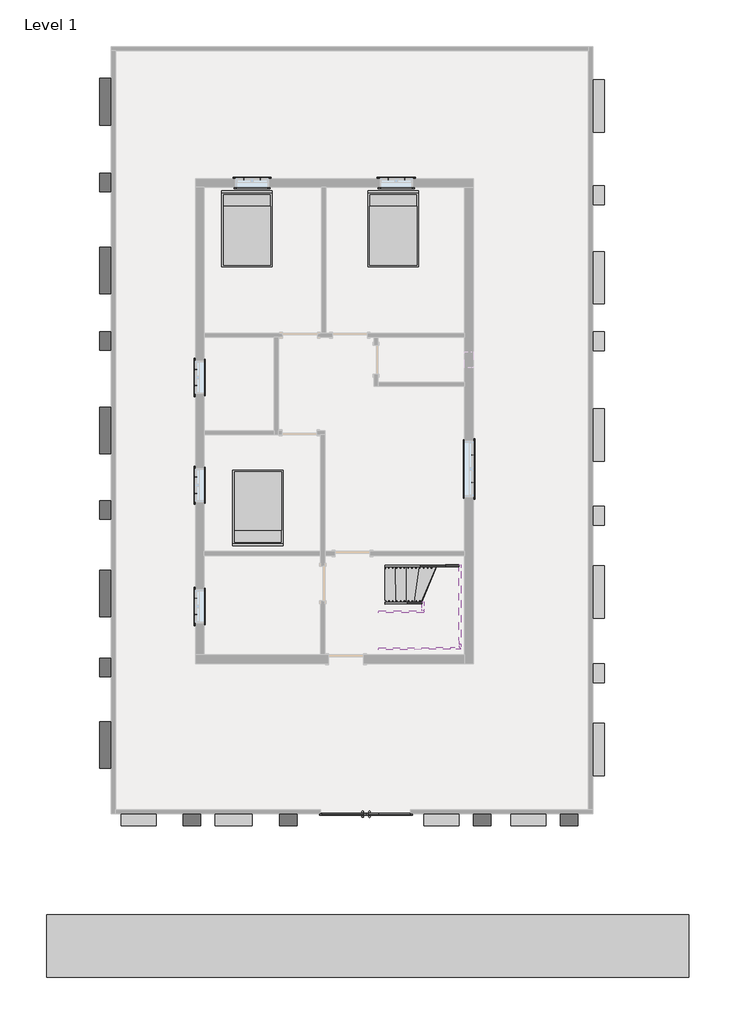
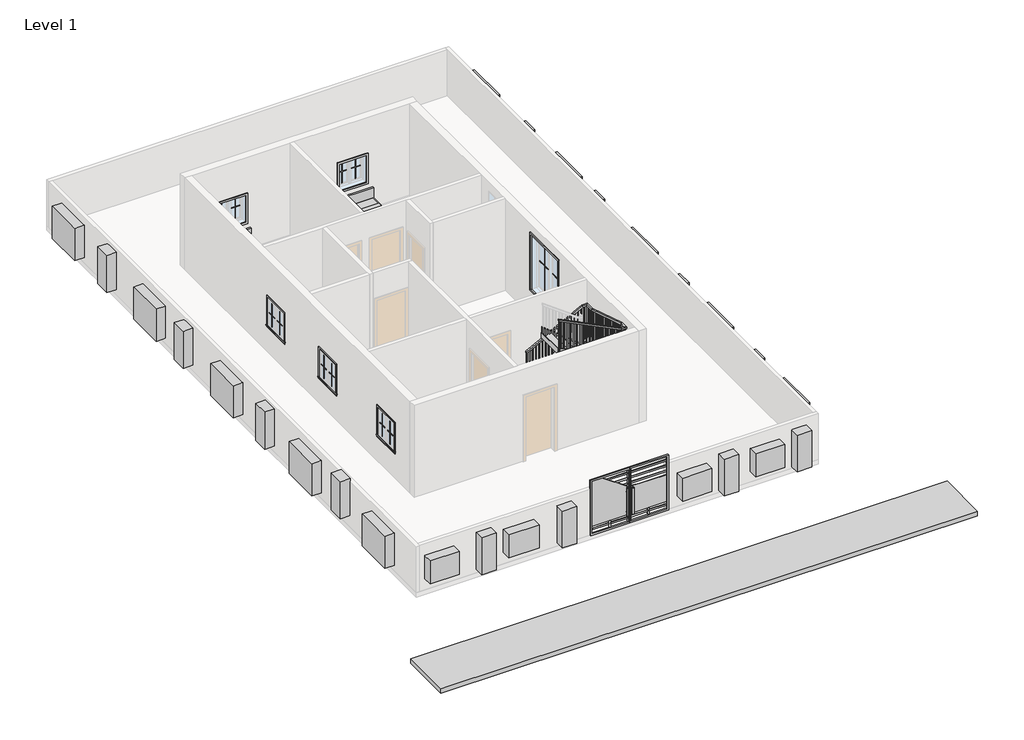
# One storey, part 2 of 2: 30 proxies, 9 members, 3 furniture elements, 1 railing, 1 stair flight.
"""IFC4 building model written with IfcOpenShell, lengths in millimetres."""

from ifc_helpers import new_model, si_unit, frame, origin, place, context, project, spatial, polyline, outline, extrude, faceted_brep, transform, mapped, element, save
from components import generic_models_113f6068, generic_models_1_generic_models_1_f3bdfb45, generic_models_2_generic_models_2_eb82d3b8, generic_models_3_generic_models_3_98a77e8e, generic_models_4_generic_models_4_94af110e, generic_models_6_generic_models_6_790b48f3, muntin_pattern_2x2_muntin_pattern_2x2_b3fe6957, muntin_pattern_2x2_muntin_pattern_2x2_3e0ecaf2, muntin_pattern_2x2_muntin_pattern_2x2_bff912c5, muntin_pattern_2x2_muntin_pattern_2x2_c2194282, trim_window_exterior_flat_with_sill_41619996, trim_window_exterior_flat_with_sill_e04b3088, trim_window_interior_flat_picture_frame_51c85655, trim_window_interior_flat_picture_frame_2a7685fe, bed_17739_bed_17739_15c61121, stair_flight_2f6b2362

model = new_model("IFC4")

# Units and contexts
model_context = context("Model", 3, world=origin())
ifc_project = project(units=[si_unit("LENGTHUNIT", "METRE", prefix="MILLI")], contexts=[model_context])

# Site, building, storey
site = spatial("IfcSite", under=ifc_project)
building = spatial("IfcBuilding", under=site)
storey = spatial("IfcBuildingStorey", under=building, Name="Level 1", Elevation=0.0)

# Proxies
placement = place(None, origin())
generic_models_shape = generic_models_113f6068(model_context)
element("IfcBuildingElementProxy", 1, Name="Generic Models", at=placement, inside=storey, context=model_context, shape_type="MappedRepresentation", body=[
    mapped(generic_models_shape, transform((-423.3915084, -9726.243996, 0.0), x_axis=(1.0, 0.0, 0.0), y_axis=(0.0, 1.0, 0.0), z_axis=(0.0, 0.0, 1.0))),
])
generic_models_1_generic_models_1_shape = generic_models_1_generic_models_1_f3bdfb45(model_context)
element("IfcBuildingElementProxy", 2, Name="Generic Models 1 : Generic Models 1", ObjectType="Generic Models 1 : Generic Models 1", at=placement, inside=storey, context=model_context, shape_type="MappedRepresentation", body=[
    mapped(generic_models_1_generic_models_1_shape, transform((0.0, 0.0, 0.0), x_axis=(1.0, 0.0, 0.0), y_axis=(0.0, 1.0, 0.0), z_axis=(0.0, 0.0, 1.0))),
])
generic_models_2_generic_models_2_shape = generic_models_2_generic_models_2_eb82d3b8(model_context)
element("IfcBuildingElementProxy", 3, Name="Generic Models 2 : Generic Models 2", ObjectType="Generic Models 2 : Generic Models 2", at=placement, inside=storey, context=model_context, shape_type="MappedRepresentation", body=[
    mapped(generic_models_2_generic_models_2_shape, transform((0.0, 0.0, 0.0), x_axis=(1.0, 0.0, 0.0), y_axis=(0.0, 1.0, 0.0), z_axis=(0.0, 0.0, 1.0))),
])
generic_models_3_generic_models_3_shape = generic_models_3_generic_models_3_98a77e8e(model_context)
element("IfcBuildingElementProxy", 4, Name="Generic Models 3 : Generic Models 3", ObjectType="Generic Models 3 : Generic Models 3", at=placement, inside=storey, context=model_context, shape_type="MappedRepresentation", body=[
    mapped(generic_models_3_generic_models_3_shape, transform((0.0, 0.0, 0.0), x_axis=(1.0, 0.0, 0.0), y_axis=(0.0, 1.0, 0.0), z_axis=(0.0, 0.0, 1.0))),
])
generic_models_4_generic_models_4_shape = generic_models_4_generic_models_4_94af110e(model_context)
element("IfcBuildingElementProxy", 5, Name="Generic Models 4 : Generic Models 4", ObjectType="Generic Models 4 : Generic Models 4", at=placement, inside=storey, context=model_context, shape_type="MappedRepresentation", body=[
    mapped(generic_models_4_generic_models_4_shape, transform((0.0, 0.0, 0.0), x_axis=(1.0, 0.0, 0.0), y_axis=(0.0, 1.0, 0.0), z_axis=(0.0, 0.0, 1.0))),
])
generic_models_6_generic_models_6_shape = generic_models_6_generic_models_6_790b48f3(model_context)
element("IfcBuildingElementProxy", 6, Name="Generic Models 6 : Generic Models 6", ObjectType="Generic Models 6 : Generic Models 6", at=placement, inside=storey, context=model_context, shape_type="MappedRepresentation", body=[
    mapped(generic_models_6_generic_models_6_shape, transform((0.0, 0.0, 0.0), x_axis=(1.0, 0.0, 0.0), y_axis=(0.0, 1.0, 0.0), z_axis=(0.0, 0.0, 1.0))),
])
muntin_pattern_2x2_muntin_pattern_2x2_shape = muntin_pattern_2x2_muntin_pattern_2x2_b3fe6957(model_context)
element("IfcBuildingElementProxy", 7, Name="Muntin Pattern_2x2 : Muntin Pattern_2x2", ObjectType="Muntin Pattern_2x2 : Muntin Pattern_2x2", at=placement, inside=storey, context=model_context, shape_type="MappedRepresentation", body=[
    mapped(muntin_pattern_2x2_muntin_pattern_2x2_shape, transform((-3622.2040084, 6872.3185985, 984.25), x_axis=(1.0, 0.0, 0.0), y_axis=(0.0, 1.0, 0.0), z_axis=(0.0, 0.0, 1.0))),
])
element("IfcBuildingElementProxy", 8, Name="Muntin Pattern_2x2 : Muntin Pattern_2x2", ObjectType="Muntin Pattern_2x2 : Muntin Pattern_2x2", at=placement, inside=storey, context=model_context, shape_type="MappedRepresentation", body=[
    mapped(muntin_pattern_2x2_muntin_pattern_2x2_shape, transform((152.8709916, 6872.3185985, 984.25), x_axis=(1.0, 0.0, 0.0), y_axis=(0.0, 1.0, 0.0), z_axis=(0.0, 0.0, 1.0))),
])
element("IfcBuildingElementProxy", 9, Name="Muntin Pattern_2x2 : Muntin Pattern_2x2", ObjectType="Muntin Pattern_2x2 : Muntin Pattern_2x2", at=placement, inside=storey, context=model_context, shape_type="MappedRepresentation", body=[
    mapped(muntin_pattern_2x2_muntin_pattern_2x2_shape, transform((-4884.2665084, 1466.8810985, 984.25), x_axis=(0.0, 1.0, 0.0), y_axis=(-1.0, 0.0, 0.0), z_axis=(0.0, 0.0, 1.0))),
])
element("IfcBuildingElementProxy", 10, Name="Muntin Pattern_2x2 : Muntin Pattern_2x2", ObjectType="Muntin Pattern_2x2 : Muntin Pattern_2x2", at=placement, inside=storey, context=model_context, shape_type="MappedRepresentation", body=[
    mapped(muntin_pattern_2x2_muntin_pattern_2x2_shape, transform((-4884.2665084, -1352.5189015, 984.25), x_axis=(0.0, 1.0, 0.0), y_axis=(-1.0, 0.0, 0.0), z_axis=(0.0, 0.0, 1.0))),
])
element("IfcBuildingElementProxy", 11, Name="Muntin Pattern_2x2 : Muntin Pattern_2x2", ObjectType="Muntin Pattern_2x2 : Muntin Pattern_2x2", at=placement, inside=storey, context=model_context, shape_type="MappedRepresentation", body=[
    mapped(muntin_pattern_2x2_muntin_pattern_2x2_shape, transform((-4884.2665084, -4524.3439015, 984.25), x_axis=(0.0, 1.0, 0.0), y_axis=(-1.0, 0.0, 0.0), z_axis=(0.0, 0.0, 1.0))),
])
muntin_pattern_2x2_muntin_pattern_2x2_2_shape = muntin_pattern_2x2_muntin_pattern_2x2_3e0ecaf2(model_context)
element("IfcBuildingElementProxy", 12, Name="Muntin Pattern_2x2 : Muntin Pattern_2x2", ObjectType="Muntin Pattern_2x2 : Muntin Pattern_2x2", at=placement, inside=storey, context=model_context, shape_type="MappedRepresentation", body=[
    mapped(muntin_pattern_2x2_muntin_pattern_2x2_2_shape, transform((-3193.5790084, 6872.3185985, 984.25), x_axis=(-1.0, 0.0, 0.0), y_axis=(0.0, -1.0, 0.0), z_axis=(0.0, 0.0, 1.0))),
])
element("IfcBuildingElementProxy", 13, Name="Muntin Pattern_2x2 : Muntin Pattern_2x2", ObjectType="Muntin Pattern_2x2 : Muntin Pattern_2x2", at=placement, inside=storey, context=model_context, shape_type="MappedRepresentation", body=[
    mapped(muntin_pattern_2x2_muntin_pattern_2x2_2_shape, transform((581.4959916, 6872.3185985, 984.25), x_axis=(-1.0, 0.0, 0.0), y_axis=(0.0, -1.0, 0.0), z_axis=(0.0, 0.0, 1.0))),
])
element("IfcBuildingElementProxy", 14, Name="Muntin Pattern_2x2 : Muntin Pattern_2x2", ObjectType="Muntin Pattern_2x2 : Muntin Pattern_2x2", at=placement, inside=storey, context=model_context, shape_type="MappedRepresentation", body=[
    mapped(muntin_pattern_2x2_muntin_pattern_2x2_2_shape, transform((-4884.2665084, 1895.5060985, 984.25), x_axis=(0.0, -1.0, 0.0), y_axis=(1.0, 0.0, 0.0), z_axis=(0.0, 0.0, 1.0))),
])
element("IfcBuildingElementProxy", 15, Name="Muntin Pattern_2x2 : Muntin Pattern_2x2", ObjectType="Muntin Pattern_2x2 : Muntin Pattern_2x2", at=placement, inside=storey, context=model_context, shape_type="MappedRepresentation", body=[
    mapped(muntin_pattern_2x2_muntin_pattern_2x2_2_shape, transform((-4884.2665084, -923.8939015, 984.25), x_axis=(0.0, -1.0, 0.0), y_axis=(1.0, 0.0, 0.0), z_axis=(0.0, 0.0, 1.0))),
])
element("IfcBuildingElementProxy", 16, Name="Muntin Pattern_2x2 : Muntin Pattern_2x2", ObjectType="Muntin Pattern_2x2 : Muntin Pattern_2x2", at=placement, inside=storey, context=model_context, shape_type="MappedRepresentation", body=[
    mapped(muntin_pattern_2x2_muntin_pattern_2x2_2_shape, transform((-4884.2665084, -4095.7189015, 984.25), x_axis=(0.0, -1.0, 0.0), y_axis=(1.0, 0.0, 0.0), z_axis=(0.0, 0.0, 1.0))),
])
muntin_pattern_2x2_muntin_pattern_2x2_3_shape = muntin_pattern_2x2_muntin_pattern_2x2_bff912c5(model_context)
element("IfcBuildingElementProxy", 17, Name="Muntin Pattern_2x2 : Muntin Pattern_2x2", ObjectType="Muntin Pattern_2x2 : Muntin Pattern_2x2", at=placement, inside=storey, context=model_context, shape_type="MappedRepresentation", body=[
    mapped(muntin_pattern_2x2_muntin_pattern_2x2_3_shape, transform((2373.7834916, -352.3939015, 984.25), x_axis=(0.0, -1.0, 0.0), y_axis=(1.0, 0.0, 0.0), z_axis=(0.0, 0.0, 1.0))),
])
muntin_pattern_2x2_muntin_pattern_2x2_4_shape = muntin_pattern_2x2_muntin_pattern_2x2_c2194282(model_context)
element("IfcBuildingElementProxy", 18, Name="Muntin Pattern_2x2 : Muntin Pattern_2x2", ObjectType="Muntin Pattern_2x2 : Muntin Pattern_2x2", at=placement, inside=storey, context=model_context, shape_type="MappedRepresentation", body=[
    mapped(muntin_pattern_2x2_muntin_pattern_2x2_4_shape, transform((2373.7834916, -1073.1189015, 984.25), x_axis=(0.0, 1.0, 0.0), y_axis=(-1.0, 0.0, 0.0), z_axis=(0.0, 0.0, 1.0))),
])
trim_window_exterior_flat_with_sill_shape = trim_window_exterior_flat_with_sill_41619996(model_context)
element("IfcBuildingElementProxy", 19, Name="Trim-Window-Exterior-Flat : with Sill", ObjectType="Trim-Window-Exterior-Flat : with Sill", at=placement, inside=storey, context=model_context, shape_type="MappedRepresentation", body=[
    mapped(trim_window_exterior_flat_with_sill_shape, transform((-3407.8915084, 6881.8435985, 1828.8), x_axis=(-1.0, 0.0, 0.0), y_axis=(0.0, 0.0, 1.0), z_axis=(0.0, 1.0, 0.0))),
])
element("IfcBuildingElementProxy", 20, Name="Trim-Window-Exterior-Flat : with Sill", ObjectType="Trim-Window-Exterior-Flat : with Sill", at=placement, inside=storey, context=model_context, shape_type="MappedRepresentation", body=[
    mapped(trim_window_exterior_flat_with_sill_shape, transform((367.1834916, 6881.8435985, 1828.8), x_axis=(-1.0, 0.0, 0.0), y_axis=(0.0, 0.0, 1.0), z_axis=(0.0, 1.0, 0.0))),
])
element("IfcBuildingElementProxy", 21, Name="Trim-Window-Exterior-Flat : with Sill", ObjectType="Trim-Window-Exterior-Flat : with Sill", at=placement, inside=storey, context=model_context, shape_type="MappedRepresentation", body=[
    mapped(trim_window_exterior_flat_with_sill_shape, transform((-4893.7915084, 1681.1935985, 1828.8), x_axis=(0.0, -1.0, 0.0), y_axis=(0.0, 0.0, 1.0), z_axis=(-1.0, 0.0, 0.0))),
])
element("IfcBuildingElementProxy", 22, Name="Trim-Window-Exterior-Flat : with Sill", ObjectType="Trim-Window-Exterior-Flat : with Sill", at=placement, inside=storey, context=model_context, shape_type="MappedRepresentation", body=[
    mapped(trim_window_exterior_flat_with_sill_shape, transform((-4893.7915084, -1138.2064015, 1828.8), x_axis=(0.0, -1.0, 0.0), y_axis=(0.0, 0.0, 1.0), z_axis=(-1.0, 0.0, 0.0))),
])
element("IfcBuildingElementProxy", 23, Name="Trim-Window-Exterior-Flat : with Sill", ObjectType="Trim-Window-Exterior-Flat : with Sill", at=placement, inside=storey, context=model_context, shape_type="MappedRepresentation", body=[
    mapped(trim_window_exterior_flat_with_sill_shape, transform((-4893.7915084, -4310.0314015, 1828.8), x_axis=(0.0, -1.0, 0.0), y_axis=(0.0, 0.0, 1.0), z_axis=(-1.0, 0.0, 0.0))),
])
trim_window_exterior_flat_with_sill_2_shape = trim_window_exterior_flat_with_sill_e04b3088(model_context)
element("IfcBuildingElementProxy", 24, Name="Trim-Window-Exterior-Flat : with Sill", ObjectType="Trim-Window-Exterior-Flat : with Sill", at=placement, inside=storey, context=model_context, shape_type="MappedRepresentation", body=[
    mapped(trim_window_exterior_flat_with_sill_2_shape, transform((2383.3084916, -712.7564015, 2743.2), x_axis=(0.0, 1.0, 0.0), y_axis=(0.0, 0.0, 1.0), z_axis=(1.0, 0.0, 0.0))),
])
trim_window_interior_flat_picture_frame_shape = trim_window_interior_flat_picture_frame_51c85655(model_context)
element("IfcBuildingElementProxy", 25, Name="Trim-Window-Interior-Flat : Picture Frame", ObjectType="Trim-Window-Interior-Flat : Picture Frame", at=placement, inside=storey, context=model_context, shape_type="MappedRepresentation", body=[
    mapped(trim_window_interior_flat_picture_frame_shape, transform((-3407.8915084, 6653.2435985, 1828.8), x_axis=(1.0, 0.0, 0.0), y_axis=(0.0, 0.0, 1.0), z_axis=(0.0, -1.0, 0.0))),
])
element("IfcBuildingElementProxy", 26, Name="Trim-Window-Interior-Flat : Picture Frame", ObjectType="Trim-Window-Interior-Flat : Picture Frame", at=placement, inside=storey, context=model_context, shape_type="MappedRepresentation", body=[
    mapped(trim_window_interior_flat_picture_frame_shape, transform((367.1834916, 6653.2435985, 1828.8), x_axis=(1.0, 0.0, 0.0), y_axis=(0.0, 0.0, 1.0), z_axis=(0.0, -1.0, 0.0))),
])
element("IfcBuildingElementProxy", 27, Name="Trim-Window-Interior-Flat : Picture Frame", ObjectType="Trim-Window-Interior-Flat : Picture Frame", at=placement, inside=storey, context=model_context, shape_type="MappedRepresentation", body=[
    mapped(trim_window_interior_flat_picture_frame_shape, transform((-4665.1915084, 1681.1935985, 1828.8), x_axis=(0.0, 1.0, 0.0), y_axis=(0.0, 0.0, 1.0), z_axis=(1.0, 0.0, 0.0))),
])
element("IfcBuildingElementProxy", 28, Name="Trim-Window-Interior-Flat : Picture Frame", ObjectType="Trim-Window-Interior-Flat : Picture Frame", at=placement, inside=storey, context=model_context, shape_type="MappedRepresentation", body=[
    mapped(trim_window_interior_flat_picture_frame_shape, transform((-4665.1915084, -1138.2064015, 1828.8), x_axis=(0.0, 1.0, 0.0), y_axis=(0.0, 0.0, 1.0), z_axis=(1.0, 0.0, 0.0))),
])
element("IfcBuildingElementProxy", 29, Name="Trim-Window-Interior-Flat : Picture Frame", ObjectType="Trim-Window-Interior-Flat : Picture Frame", at=placement, inside=storey, context=model_context, shape_type="MappedRepresentation", body=[
    mapped(trim_window_interior_flat_picture_frame_shape, transform((-4665.1915084, -4310.0314015, 1828.8), x_axis=(0.0, 1.0, 0.0), y_axis=(0.0, 0.0, 1.0), z_axis=(1.0, 0.0, 0.0))),
])
trim_window_interior_flat_picture_frame_2_shape = trim_window_interior_flat_picture_frame_2a7685fe(model_context)
element("IfcBuildingElementProxy", 30, Name="Trim-Window-Interior-Flat : Picture Frame", ObjectType="Trim-Window-Interior-Flat : Picture Frame", at=placement, inside=storey, context=model_context, shape_type="MappedRepresentation", body=[
    mapped(trim_window_interior_flat_picture_frame_2_shape, transform((2154.7084916, -712.7564015, 2743.2), x_axis=(0.0, -1.0, 0.0), y_axis=(0.0, 0.0, 1.0), z_axis=(-1.0, 0.0, 0.0))),
])

# Furniture
bed_17739_bed_17739_shape = bed_17739_bed_17739_15c61121(model_context)
element("IfcFurniture", 31, ObjectType="Bed_17739 : Bed_17739", at=placement, inside=storey, context=model_context, shape_type="MappedRepresentation", body=[
    mapped(bed_17739_bed_17739_shape, transform((-3541.2415084, 5548.3435985, 0.0), x_axis=(1.0, 0.0, 0.0), y_axis=(0.0, 1.0, 0.0), z_axis=(0.0, 0.0, 1.0))),
])
element("IfcFurniture", 32, ObjectType="Bed_17739 : Bed_17739", at=placement, inside=storey, context=model_context, shape_type="MappedRepresentation", body=[
    mapped(bed_17739_bed_17739_shape, transform((287.8084916, 5548.3435985, 0.0), x_axis=(1.0, 0.0, 0.0), y_axis=(0.0, 1.0, 0.0), z_axis=(0.0, 0.0, 1.0))),
])
element("IfcFurniture", 33, ObjectType="Bed_17739 : Bed_17739", at=placement, inside=storey, context=model_context, shape_type="MappedRepresentation", body=[
    mapped(bed_17739_bed_17739_shape, transform((-3255.4915084, -1709.7064015, 0.0), x_axis=(-1.0, 0.0, 0.0), y_axis=(0.0, -1.0, 0.0), z_axis=(0.0, 0.0, 1.0))),
])

# Members
element("IfcMember", 34, ObjectType="Stringer - 2\" Width", at=placement, inside=storey, context=model_context, shape_type="SweptSolid", body=[
    extrude(outline(polyline([(149.3129896, -304.8), (0.0, 0.0), (1768.8429208, 0.0), (1918.1559104, -304.8000001), (149.3129896, -304.8)])), frame((68.8012135, -3282.7418259, 403.3997735), z_axis=(-0.005162073969671616, 0.9999866764074068, 0.0), x_axis=(0.8980237466183224, 0.004635726771100306, 0.4399225619889198)), (0.0, 0.0, 1.0), 50.8),
])
element("IfcMember", 35, ObjectType="Stringer - 2\" Width", at=placement, inside=storey, context=model_context, shape_type="SweptSolid", body=[
    extrude(outline(polyline([(1657.2641604, -3274.5419534), (1657.0019271, -3223.7426303), (2003.5241973, -3221.9538329), (2003.7864306, -3272.753156), (1657.2641604, -3274.5419534)])), frame((0.0, 0.0, 1181.553683), z_axis=(0.0, 0.0, 1.0), x_axis=(1.0, 0.0, 0.0)), (0.0, 0.0, 1.0), 339.4074379),
])
element("IfcMember", 36, ObjectType="Stringer - 2\" Width", at=placement, inside=storey, context=model_context, shape_type="SweptSolid", body=[
    extrude(outline(polyline([(47.2049979, -324.2228076), (-38.2916769, -48.0839082), (117.0107078, 0.0), (2125.7436964, 0.0), (2226.1278582, -324.2228076), (47.2049979, -324.2228076)])), frame((2003.7864306, -3272.753156, 1181.553683), z_axis=(0.9999866764074068, 0.00516207396967178, 0.0), x_axis=(0.004931129753271636, -0.9552486233011706, 0.29576299910667453)), (0.0, 0.0, 1.0), 50.8),
])
element("IfcMember", 37, ObjectType="Stringer - 2\" Width", at=placement, inside=storey, context=model_context, shape_type="SweptSolid", body=[
    extrude(outline(polyline([(2014.2687486, -5303.3668955), (2065.0680718, -5303.1046621), (2065.7306715, -5431.462157), (2014.669115, -5380.9250672), (2014.2687486, -5303.3668955)])), frame((0.0, 0.0, 1820.2291102), z_axis=(0.0, 0.0, 1.0), x_axis=(1.0, 0.0, 0.0)), (0.0, 0.0, 1.0), 319.0749838),
])
element("IfcMember", 38, ObjectType="Stringer - 2\" Width", at=placement, inside=storey, context=model_context, shape_type="SweptSolid", body=[
    extrude(outline(polyline([(2014.669115, -5380.9250672), (2065.7306715, -5431.462157), (1782.4368375, -5432.9245602), (1782.1746041, -5382.1252371), (2014.669115, -5380.9250672)])), frame((0.0, 0.0, 1820.2291102), z_axis=(0.0, 0.0, 1.0), x_axis=(1.0, 0.0, 0.0)), (0.0, 0.0, 1.0), 319.0749838),
])
element("IfcMember", 39, ObjectType="Stringer - 2\" Width", at=placement, inside=storey, context=model_context, shape_type="SweptSolid", body=[
    extrude(outline(polyline([(286.8047106, -304.8), (0.0, 0.0), (1331.6484515, 0.0), (1618.4531621, -304.8), (286.8047106, -304.8)])), frame((73.7836473, -4247.928966, 246.5616111), z_axis=(-0.005162073969671482, 0.9999866764074068, 0.0), x_axis=(0.7282688430294203, 0.0037594277266083495, 0.6852812261953176)), (0.0, 0.0, 1.0), 50.8),
])
element("IfcMember", 40, ObjectType="Stringer - 2\" Width", at=placement, inside=storey, context=model_context, shape_type="SweptSolid", body=[
    extrude(outline(polyline([(660.780085, -304.8), (110.7389009, -51.080863), (134.3011229, 0.0), (545.7678218, 0.0), (1125.9670058, -267.6302075), (1108.8215849, -304.8), (660.780085, -304.8)])), frame((1043.319491, -4192.1234067, 1084.9637993), z_axis=(0.9999866764074069, 0.005162073969671281, 0.0), x_axis=(0.002162183372020067, -0.4188538515087166, 0.9080510866902697)), (0.0, 0.0, 1.0), 50.8),
])
element("IfcMember", 41, ObjectType="Stringer - 2\" Width", at=placement, inside=storey, context=model_context, shape_type="SweptSolid", body=[
    extrude(outline(polyline([(-239.6623642, -304.8), (0.0, 0.0), (1521.9461582, 0.0), (1282.2837939, -304.8), (-239.6623642, -304.8)])), frame((1095.5610976, -4471.2574507, 2219.4987993), z_axis=(-0.005162073969672185, 0.9999866764074068, 0.0), x_axis=(-0.7860864868637555, -0.004057890657432356, 0.6181032023000781)), (0.0, 0.0, 1.0), 50.8),
])
element("IfcMember", 42, ObjectType="Stringer - 2\" Width", at=placement, inside=storey, context=model_context, shape_type="SweptSolid", body=[
    extrude(outline(polyline([(-137.2719745, -288.0368905), (0.0, 0.0), (2080.7002403, 0.0), (1943.4282658, -288.0368905), (-137.2719745, -288.0368905)])), frame((1782.4368375, -5432.9245602, 2139.304094), z_axis=(-0.005162073969671803, 0.9999866764074069, 0.0), x_axis=(-0.9027127399072911, -0.004659932023802336, 0.4302185424207158)), (0.0, 0.0, 1.0), 50.8),
])

# Railing
element("IfcRailing", 43, ObjectType="Handrail - Rectangular", at=placement, inside=storey, context=model_context, shape_type="SolidModel", body=[
    faceted_brep([(68.8012135, -3282.7418259, 1591.7333333), (68.8012135, -3282.7418259, 1534.6032367), (69.0634468, -3333.5411491, 1534.6032367), (69.0634468, -3333.5411491, 1591.7333333), (1818.9474855, -3273.707321, 2492.2523232), (1831.2499413, -3273.643814, 2441.4523232), (1831.5121746, -3324.4431372, 2441.4523232), (1819.2097188, -3324.5066442, 2492.2523232), (2003.7864306, -3272.753156, 2492.2523232), (2003.7864306, -3272.753156, 2441.4523232), (1953.2493408, -3323.8147125, 2441.4523232), (1953.2493408, -3323.8147125, 2492.2523232), (2005.285328, -3563.1165554, 2492.2523232), (2005.3249947, -3570.8007251, 2441.4523232), (1954.5256716, -3571.0629585, 2441.4523232), (1954.4860048, -3563.3787887, 2492.2523232), (2013.5123671, -5156.842168, 2985.6998462), (2013.5520339, -5164.5263378, 2934.8998462), (1962.7527107, -5164.7885712, 2934.8998462), (1962.7130439, -5157.1044014, 2985.6998462), (2014.669115, -5380.9250672, 2985.6998462), (2014.669115, -5380.9250672, 2934.8998462), (1963.6075585, -5330.3879774, 2934.8998462), (1963.6075585, -5330.3879774, 2985.6998462), (1865.7077622, -5381.694027, 2985.6998462), (1853.7618085, -5381.7556937, 2934.8998462), (1853.4995752, -5330.9563705, 2934.8998462), (1865.4455288, -5330.8947038, 2985.6998462), (-96.1000106, -5391.8211588, 3962.4), (-96.362244, -5341.0218356, 3962.4), (-96.362244, -5341.0218356, 3905.6526208), (-96.1000106, -5391.8211588, 3905.6526208)], [[[0, 1, 2, 3]], [[1, 0, 4, 5]], [[2, 1, 5, 6]], [[3, 2, 6, 7]], [[0, 3, 7, 4]], [[5, 4, 8, 9]], [[6, 5, 9, 10]], [[7, 6, 10, 11]], [[4, 7, 11, 8]], [[9, 8, 12, 13]], [[10, 9, 13, 14]], [[11, 10, 14, 15]], [[8, 11, 15, 12]], [[13, 12, 16, 17]], [[14, 13, 17, 18]], [[15, 14, 18, 19]], [[12, 15, 19, 16]], [[17, 16, 20, 21]], [[18, 17, 21, 22]], [[19, 18, 22, 23]], [[16, 19, 23, 20]], [[21, 20, 24, 25]], [[22, 21, 25, 26]], [[23, 22, 26, 27]], [[20, 23, 27, 24]], [[28, 29, 30, 31]], [[25, 24, 28, 31]], [[26, 25, 31, 30]], [[27, 26, 30, 29]], [[24, 27, 29, 28]]]),
    extrude(outline(polyline([(223.8579732, 19.05), (1229.0021026, 19.05), (1229.0021026, 0.0), (233.3420268, 0.0), (223.8579732, 19.05)])), frame((-33.2605479, -5375.621561, 4107.6687693), z_axis=(-0.005162073969671937, 0.9999866764074068, 0.0), x_axis=(0.0, 0.0, -1.0)), (0.0, 0.0, 1.0), 19.05),
    extrude(outline(polyline([(223.8579732, 19.0499999), (1178.4204835, 19.0499999), (1178.4204835, 0.0), (233.3420268, 0.0), (223.8579732, 19.0499999)])), frame((68.3380984, -5375.0970942, 4057.0871502), z_axis=(-0.005162073969671937, 0.9999866764074068, 0.0), x_axis=(0.0, 0.0, -1.0)), (0.0, 0.0, 1.0), 19.05),
    extrude(outline(polyline([(223.8579732, 19.05), (1127.8388644, 19.05), (1127.8388644, 0.0), (233.3420268, 0.0), (223.8579732, 19.05)])), frame((169.9367448, -5374.5726275, 4006.5055311), z_axis=(-0.005162073969671937, 0.9999866764074068, 0.0), x_axis=(0.0, 0.0, -1.0)), (0.0, 0.0, 1.0), 19.05),
    extrude(outline(polyline([(223.8579732, 19.05), (1246.5905787, 19.05), (1246.5905787, 0.0), (233.3420268, 0.0), (223.8579732, 19.05)])), frame((271.5353911, -5374.0481608, 3955.923912), z_axis=(-0.005162073969671937, 0.9999866764074068, 0.0), x_axis=(0.0, 0.0, -1.0)), (0.0, 0.0, 1.0), 19.05),
    extrude(outline(polyline([(223.8579732, 19.05), (1196.0089596, 19.05), (1196.0089596, 0.0), (233.3420267, 0.0), (223.8579732, 19.05)])), frame((373.1340374, -5373.5236941, 3905.3422929), z_axis=(-0.005162073969671937, 0.9999866764074068, 0.0), x_axis=(0.0, 0.0, -1.0)), (0.0, 0.0, 1.0), 19.05),
    extrude(outline(polyline([(223.8579732, 19.05), (1314.7606738, 19.05), (1314.7606738, 0.0), (233.3420267, 0.0), (223.8579732, 19.05)])), frame((474.7326837, -5372.9992274, 3854.7606738), z_axis=(-0.005162073969671937, 0.9999866764074068, 0.0), x_axis=(0.0, 0.0, -1.0)), (0.0, 0.0, 1.0), 19.05),
    extrude(outline(polyline([(223.8579733, 19.05), (1264.1790548, 19.05), (1264.1790548, 0.0), (233.3420268, 0.0), (223.8579733, 19.05)])), frame((576.3313301, -5372.4747607, 3804.1790548), z_axis=(-0.005162073969671937, 0.9999866764074068, 0.0), x_axis=(0.0, 0.0, -1.0)), (0.0, 0.0, 1.0), 19.05),
    extrude(outline(polyline([(223.8579732, 19.05), (1213.5974357, 19.05), (1213.5974357, 0.0), (233.3420268, 0.0), (223.8579732, 19.05)])), frame((677.9299764, -5371.950294, 3753.5974357), z_axis=(-0.005162073969671937, 0.9999866764074068, 0.0), x_axis=(0.0, 0.0, -1.0)), (0.0, 0.0, 1.0), 19.05),
    extrude(outline(polyline([(223.8579732, 19.05), (1163.0158166, 19.05), (1163.0158166, 0.0), (233.3420268, 0.0), (223.8579732, 19.05)])), frame((779.5286227, -5371.4258272, 3703.0158166), z_axis=(-0.005162073969671937, 0.9999866764074068, 0.0), x_axis=(0.0, 0.0, -1.0)), (0.0, 0.0, 1.0), 19.05),
    extrude(outline(polyline([(223.8579732, 19.05), (1281.7675308, 19.05), (1281.7675308, 0.0), (233.3420268, 0.0), (223.8579732, 19.05)])), frame((881.127269, -5370.9013605, 3652.4341975), z_axis=(-0.005162073969671937, 0.9999866764074068, 0.0), x_axis=(0.0, 0.0, -1.0)), (0.0, 0.0, 1.0), 19.05),
    extrude(outline(polyline([(223.8579732, 19.0499999), (1231.1859117, 19.0499999), (1231.1859117, 0.0), (233.3420268, 0.0), (223.8579732, 19.0499999)])), frame((982.7259153, -5370.3768938, 3601.8525784), z_axis=(-0.005162073969671937, 0.9999866764074068, 0.0), x_axis=(0.0, 0.0, -1.0)), (0.0, 0.0, 1.0), 19.05),
    extrude(outline(polyline([(223.8579732, 19.05), (1180.6042926, 19.05), (1180.6042926, 0.0), (233.3420268, 0.0), (223.8579732, 19.05)])), frame((1084.3245617, -5369.8524271, 3551.2709593), z_axis=(-0.005162073969671937, 0.9999866764074068, 0.0), x_axis=(0.0, 0.0, -1.0)), (0.0, 0.0, 1.0), 19.05),
    extrude(outline(polyline([(223.8579732, 19.05), (1299.3560069, 19.05), (1299.3560069, 0.0), (233.3420268, 0.0), (223.8579732, 19.05)])), frame((1185.923208, -5369.3279604, 3500.6893402), z_axis=(-0.005162073969671937, 0.9999866764074068, 0.0), x_axis=(0.0, 0.0, -1.0)), (0.0, 0.0, 1.0), 19.05),
    extrude(outline(polyline([(223.8579732, 19.05), (1248.7743878, 19.05), (1248.7743878, 0.0), (233.3420268, 0.0), (223.8579732, 19.05)])), frame((1287.5218543, -5368.8034937, 3450.1077211), z_axis=(-0.005162073969671937, 0.9999866764074068, 0.0), x_axis=(0.0, 0.0, -1.0)), (0.0, 0.0, 1.0), 19.05),
    extrude(outline(polyline([(223.8579732, 19.0499999), (1198.1927687, 19.0499999), (1198.1927687, 0.0), (233.3420268, 0.0), (223.8579732, 19.0499999)])), frame((1389.1205006, -5368.2790269, 3399.526102), z_axis=(-0.005162073969671937, 0.9999866764074068, 0.0), x_axis=(0.0, 0.0, -1.0)), (0.0, 0.0, 1.0), 19.05),
    extrude(outline(polyline([(223.8579732, 19.05), (1147.6111496, 19.05), (1147.6111496, 0.0), (233.3420268, 0.0), (223.8579732, 19.05)])), frame((1490.719147, -5367.7545602, 3348.9444829), z_axis=(-0.005162073969671937, 0.9999866764074068, 0.0), x_axis=(0.0, 0.0, -1.0)), (0.0, 0.0, 1.0), 19.05),
    extrude(outline(polyline([(223.8579732, 19.05), (1097.0295305, 19.05), (1097.0295305, 0.0), (233.3420267, 0.0), (223.8579732, 19.05)])), frame((1592.3177933, -5367.2300935, 3298.3628638), z_axis=(-0.005162073969671937, 0.9999866764074068, 0.0), x_axis=(0.0, 0.0, -1.0)), (0.0, 0.0, 1.0), 19.05),
    extrude(outline(polyline([(223.8579733, 19.05), (1215.7812448, 19.05), (1215.7812448, 0.0), (233.3420268, 0.0), (223.8579733, 19.05)])), frame((1693.9164396, -5366.7056268, 3247.7812448), z_axis=(-0.005162073969671937, 0.9999866764074068, 0.0), x_axis=(0.0, 0.0, -1.0)), (0.0, 0.0, 1.0), 19.05),
    extrude(outline(polyline([(223.8579733, 19.05), (1165.1996257, 19.05), (1165.1996257, 0.0), (233.3420268, 0.0), (223.8579733, 19.05)])), frame((1795.5150859, -5366.1811601, 3197.1996257), z_axis=(-0.005162073969671937, 0.9999866764074068, 0.0), x_axis=(0.0, 0.0, -1.0)), (0.0, 0.0, 1.0), 19.05),
    extrude(outline(polyline([(1897.1137323, -5365.6566934), (1878.0639861, -5365.7550309), (1877.9656486, -5346.7052847), (1897.0153947, -5346.6069472), (1897.1137323, -5365.6566934)])), frame((0.0, 0.0, 2032.0), z_axis=(0.0, 0.0, 1.0), x_axis=(1.0, 0.0, 0.0)), (0.0, 0.0, 1.0), 902.8998462),
    extrude(outline(polyline([(1998.4829244, -5320.6828189), (1998.5812619, -5339.7325651), (1979.5315157, -5339.8309026), (1979.4331782, -5320.7811564), (1998.4829244, -5320.6828189)])), frame((0.0, 0.0, 2032.0), z_axis=(0.0, 0.0, 1.0), x_axis=(1.0, 0.0, 0.0)), (0.0, 0.0, 1.0), 902.8998462),
    extrude(outline(polyline([(1997.9584577, -5219.0841726), (1998.0567952, -5238.1339187), (1979.007049, -5238.2322563), (1978.9087115, -5219.1825101), (1997.9584577, -5219.0841726)])), frame((0.0, 0.0, 2032.0), z_axis=(0.0, 0.0, 1.0), x_axis=(1.0, 0.0, 0.0)), (0.0, 0.0, 1.0), 902.8998462),
    extrude(outline(polyline([(231.5490805, 19.05), (1119.8588311, 19.05), (1119.8588311, 0.0), (225.6509196, 0.0), (231.5490805, 19.05)])), frame((1978.4825823, -5136.6336099, 3151.8588311), z_axis=(0.9999866764074068, 0.005162073969671697, 0.0), x_axis=(0.0, 0.0, -1.0)), (0.0, 0.0, 1.0), 19.05),
    extrude(outline(polyline([(231.5490804, 19.05), (1088.401973, 19.05), (1088.401973, 0.0), (225.6509195, 0.0), (231.5490804, 19.05)])), frame((1977.9581156, -5035.0349636, 3120.401973), z_axis=(0.9999866764074068, 0.005162073969671697, 0.0), x_axis=(0.0, 0.0, -1.0)), (0.0, 0.0, 1.0), 19.05),
    extrude(outline(polyline([(231.5490805, 19.05), (1226.2784483, 19.05), (1226.2784483, 0.0), (225.6509196, 0.0), (231.5490805, 19.05)])), frame((1977.4336488, -4933.4363173, 3088.945115), z_axis=(0.9999866764074068, 0.005162073969671697, 0.0), x_axis=(0.0, 0.0, -1.0)), (0.0, 0.0, 1.0), 19.05),
    extrude(outline(polyline([(231.5490804, 19.05), (1194.8215902, 19.05), (1194.8215902, 0.0), (225.6509195, 0.0), (231.5490804, 19.05)])), frame((1976.9091821, -4831.837671, 3057.4882569), z_axis=(0.9999866764074068, 0.005162073969671697, 0.0), x_axis=(0.0, 0.0, -1.0)), (0.0, 0.0, 1.0), 19.05),
    extrude(outline(polyline([(231.5490805, 19.0499999), (1163.3647322, 19.0499999), (1163.3647322, 0.0), (225.6509196, 0.0), (231.5490805, 19.0499999)])), frame((1976.3847154, -4730.2390246, 3026.0313989), z_axis=(0.9999866764074068, 0.005162073969671697, 0.0), x_axis=(0.0, 0.0, -1.0)), (0.0, 0.0, 1.0), 19.05),
    extrude(outline(polyline([(231.5490804, 19.05), (1131.9078741, 19.05), (1131.9078741, 0.0), (225.6509195, 0.0), (231.5490804, 19.05)])), frame((1975.8602487, -4628.6403783, 2994.5745408), z_axis=(0.9999866764074068, 0.005162073969671697, 0.0), x_axis=(0.0, 0.0, -1.0)), (0.0, 0.0, 1.0), 19.05),
    extrude(outline(polyline([(231.5490805, 19.05), (1100.4510161, 19.05), (1100.4510161, 0.0), (225.6509196, 0.0), (231.5490805, 19.05)])), frame((1975.335782, -4527.041732, 2963.1176828), z_axis=(0.9999866764074068, 0.005162073969671697, 0.0), x_axis=(0.0, 0.0, -1.0)), (0.0, 0.0, 1.0), 19.05),
    extrude(outline(polyline([(231.5490804, 19.05), (1238.3274914, 19.05), (1238.3274914, 0.0), (225.6509195, 0.0), (231.5490804, 19.05)])), frame((1974.8113153, -4425.4430857, 2931.6608247), z_axis=(0.9999866764074068, 0.005162073969671697, 0.0), x_axis=(0.0, 0.0, -1.0)), (0.0, 0.0, 1.0), 19.05),
    extrude(outline(polyline([(231.5490805, 19.05), (1206.8706334, 19.05), (1206.8706334, 0.0), (225.6509196, 0.0), (231.5490805, 19.05)])), frame((1974.2868486, -4323.8444394, 2900.2039667), z_axis=(0.9999866764074068, 0.005162073969671697, 0.0), x_axis=(0.0, 0.0, -1.0)), (0.0, 0.0, 1.0), 19.05),
    extrude(outline(polyline([(231.5490804, 19.05), (1175.4137753, 19.05), (1175.4137753, 0.0), (225.6509195, 0.0), (231.5490804, 19.05)])), frame((1973.7623818, -4222.245793, 2868.7471086), z_axis=(0.9999866764074068, 0.005162073969671697, 0.0), x_axis=(0.0, 0.0, -1.0)), (0.0, 0.0, 1.0), 19.05),
    extrude(outline(polyline([(231.5490804, 19.05), (1143.9569173, 19.05), (1143.9569173, 0.0), (225.6509196, 0.0), (231.5490804, 19.05)])), frame((1973.2379151, -4120.6471467, 2837.2902506), z_axis=(0.9999866764074068, 0.005162073969671697, 0.0), x_axis=(0.0, 0.0, -1.0)), (0.0, 0.0, 1.0), 19.05),
    extrude(outline(polyline([(231.5490805, 19.05), (1281.8333926, 19.05), (1281.8333926, 0.0), (225.6509196, 0.0), (231.5490805, 19.05)])), frame((1972.7134484, -4019.0485004, 2805.8333926), z_axis=(0.9999866764074068, 0.005162073969671697, 0.0), x_axis=(0.0, 0.0, -1.0)), (0.0, 0.0, 1.0), 19.05),
    extrude(outline(polyline([(231.5490804, 19.05), (1250.3765345, 19.05), (1250.3765345, 0.0), (225.6509196, 0.0), (231.5490804, 19.05)])), frame((1972.1889817, -3917.4498541, 2774.3765345), z_axis=(0.9999866764074068, 0.005162073969671697, 0.0), x_axis=(0.0, 0.0, -1.0)), (0.0, 0.0, 1.0), 19.05),
    extrude(outline(polyline([(231.5490805, 19.0499999), (1218.9196765, 19.0499999), (1218.9196765, 0.0), (225.6509196, 0.0), (231.5490805, 19.0499999)])), frame((1971.664515, -3815.8512077, 2742.9196765), z_axis=(0.9999866764074068, 0.005162073969671697, 0.0), x_axis=(0.0, 0.0, -1.0)), (0.0, 0.0, 1.0), 19.05),
    extrude(outline(polyline([(231.5490804, 19.05), (1187.4628184, 19.05), (1187.4628184, 0.0), (225.6509195, 0.0), (231.5490804, 19.05)])), frame((1971.1400483, -3714.2525614, 2711.4628184), z_axis=(0.9999866764074068, 0.005162073969671697, 0.0), x_axis=(0.0, 0.0, -1.0)), (0.0, 0.0, 1.0), 19.05),
    extrude(outline(polyline([(231.5490805, 19.05), (1156.0059604, 19.05), (1156.0059604, 0.0), (225.6509196, 0.0), (231.5490805, 19.05)])), frame((1970.6155816, -3612.6539151, 2680.0059604), z_axis=(0.9999866764074068, 0.005162073969671697, 0.0), x_axis=(0.0, 0.0, -1.0)), (0.0, 0.0, 1.0), 19.05),
    extrude(outline(polyline([(1989.0425235, -3491.9071851), (1989.140861, -3510.9569313), (1970.0911148, -3511.0552688), (1969.9927773, -3492.0055226), (1989.0425235, -3491.9071851)])), frame((0.0, 0.0, 1524.0), z_axis=(0.0, 0.0, 1.0), x_axis=(1.0, 0.0, 0.0)), (0.0, 0.0, 1.0), 917.4523232),
    extrude(outline(polyline([(1988.5180568, -3390.3085387), (1988.6163943, -3409.3582849), (1969.5666481, -3409.4566224), (1969.4683106, -3390.4068763), (1988.5180568, -3390.3085387)])), frame((0.0, 0.0, 1354.6666667), z_axis=(0.0, 0.0, 1.0), x_axis=(1.0, 0.0, 0.0)), (0.0, 0.0, 1.0), 1086.7856565),
    extrude(outline(polyline([(1888.1339221, -3289.2253823), (1907.1836683, -3289.1270448), (1907.2820058, -3308.176791), (1888.2322596, -3308.2751285), (1888.1339221, -3289.2253823)])), frame((0.0, 0.0, 1354.6666667), z_axis=(0.0, 0.0, 1.0), x_axis=(1.0, 0.0, 0.0)), (0.0, 0.0, 1.0), 1086.7856565),
    extrude(outline(polyline([(233.5009213, 19.05), (1297.2369609, 19.05), (1297.2369609, 0.0), (223.6990787, 0.0), (233.5009213, 19.05)])), frame((1805.6833595, -3308.7012577, 2651.9036276), z_axis=(-0.005162073969671542, 0.9999866764074069, 0.0), x_axis=(0.0, 0.0, -1.0)), (0.0, 0.0, 1.0), 19.05),
    extrude(outline(polyline([(233.5009213, 19.05), (1244.9604673, 19.05), (1244.9604673, 0.0), (223.6990787, 0.0), (233.5009213, 19.05)])), frame((1704.0847132, -3309.2257244, 2599.627134), z_axis=(-0.005162073969671542, 0.9999866764074069, 0.0), x_axis=(0.0, 0.0, -1.0)), (0.0, 0.0, 1.0), 19.05),
    extrude(outline(polyline([(233.5009212, 19.05), (1192.6839737, 19.05), (1192.6839737, 0.0), (223.6990787, 0.0), (233.5009212, 19.05)])), frame((1602.4860668, -3309.7501911, 2547.3506404), z_axis=(-0.005162073969671542, 0.9999866764074069, 0.0), x_axis=(0.0, 0.0, -1.0)), (0.0, 0.0, 1.0), 19.05),
    extrude(outline(polyline([(233.5009212, 19.05), (1140.4074801, 19.05), (1140.4074801, 0.0), (223.6990787, 0.0), (233.5009212, 19.05)])), frame((1500.8874205, -3310.2746578, 2495.0741468), z_axis=(-0.005162073969671542, 0.9999866764074069, 0.0), x_axis=(0.0, 0.0, -1.0)), (0.0, 0.0, 1.0), 19.05),
    extrude(outline(polyline([(233.5009213, 19.05), (1088.1309866, 19.05), (1088.1309866, 0.0), (223.6990788, 0.0), (233.5009213, 19.05)])), frame((1399.2887742, -3310.7991245, 2442.7976533), z_axis=(-0.005162073969671542, 0.9999866764074069, 0.0), x_axis=(0.0, 0.0, -1.0)), (0.0, 0.0, 1.0), 19.05),
    extrude(outline(polyline([(233.5009213, 19.05), (1205.1878264, 19.05), (1205.1878264, 0.0), (223.6990788, 0.0), (233.5009213, 19.05)])), frame((1297.6901279, -3311.3235913, 2390.5211597), z_axis=(-0.005162073969671542, 0.9999866764074069, 0.0), x_axis=(0.0, 0.0, -1.0)), (0.0, 0.0, 1.0), 19.05),
    extrude(outline(polyline([(233.5009213, 19.0499999), (1152.9113328, 19.0499999), (1152.9113328, 0.0), (223.6990787, 0.0), (233.5009213, 19.0499999)])), frame((1196.0914815, -3311.848058, 2338.2446661), z_axis=(-0.005162073969671542, 0.9999866764074069, 0.0), x_axis=(0.0, 0.0, -1.0)), (0.0, 0.0, 1.0), 19.05),
    extrude(outline(polyline([(233.5009213, 19.05), (1100.6348392, 19.05), (1100.6348392, 0.0), (223.6990787, 0.0), (233.5009213, 19.05)])), frame((1094.4928352, -3312.3725247, 2285.9681725), z_axis=(-0.005162073969671542, 0.9999866764074069, 0.0), x_axis=(0.0, 0.0, -1.0)), (0.0, 0.0, 1.0), 19.05),
    extrude(outline(polyline([(233.5009213, 19.05), (1048.3583456, 19.05), (1048.3583456, 0.0), (223.6990787, 0.0), (233.5009213, 19.05)])), frame((992.8941889, -3312.8969914, 2233.6916789), z_axis=(-0.005162073969671542, 0.9999866764074069, 0.0), x_axis=(0.0, 0.0, -1.0)), (0.0, 0.0, 1.0), 19.05),
    extrude(outline(polyline([(233.5009212, 19.05), (1165.4151853, 19.05), (1165.4151853, 0.0), (223.6990787, 0.0), (233.5009212, 19.05)])), frame((891.2955426, -3313.4214581, 2181.4151853), z_axis=(-0.005162073969671542, 0.9999866764074069, 0.0), x_axis=(0.0, 0.0, -1.0)), (0.0, 0.0, 1.0), 19.05),
    extrude(outline(polyline([(233.5009213, 19.0499999), (1113.1386918, 19.0499999), (1113.1386918, 0.0), (223.6990788, 0.0), (233.5009213, 19.0499999)])), frame((789.6968962, -3313.9459248, 2129.1386918), z_axis=(-0.005162073969671542, 0.9999866764074069, 0.0), x_axis=(0.0, 0.0, -1.0)), (0.0, 0.0, 1.0), 19.05),
    extrude(outline(polyline([(233.5009213, 19.05), (1060.8621982, 19.05), (1060.8621982, 0.0), (223.6990788, 0.0), (233.5009213, 19.05)])), frame((688.0982499, -3314.4703915, 2076.8621982), z_axis=(-0.005162073969671542, 0.9999866764074069, 0.0), x_axis=(0.0, 0.0, -1.0)), (0.0, 0.0, 1.0), 19.05),
    extrude(outline(polyline([(233.5009213, 19.05), (1177.9190379, 19.05), (1177.9190379, 0.0), (223.6990787, 0.0), (233.5009213, 19.05)])), frame((586.4996036, -3314.9948583, 2024.5857046), z_axis=(-0.005162073969671542, 0.9999866764074069, 0.0), x_axis=(0.0, 0.0, -1.0)), (0.0, 0.0, 1.0), 19.05),
    extrude(outline(polyline([(233.5009213, 19.05), (1125.6425443, 19.05), (1125.6425443, 0.0), (223.6990787, 0.0), (233.5009213, 19.05)])), frame((484.9009573, -3315.519325, 1972.309211), z_axis=(-0.005162073969671542, 0.9999866764074069, 0.0), x_axis=(0.0, 0.0, -1.0)), (0.0, 0.0, 1.0), 19.05),
    extrude(outline(polyline([(233.5009213, 19.05), (1073.3660507, 19.05), (1073.3660507, 0.0), (223.6990787, 0.0), (233.5009213, 19.05)])), frame((383.302311, -3316.0437917, 1920.0327174), z_axis=(-0.005162073969671542, 0.9999866764074069, 0.0), x_axis=(0.0, 0.0, -1.0)), (0.0, 0.0, 1.0), 19.05),
    extrude(outline(polyline([(233.5009212, 19.05), (1190.4228905, 19.05), (1190.4228905, 0.0), (223.6990787, 0.0), (233.5009212, 19.05)])), frame((281.7036646, -3316.5682584, 1867.7562238), z_axis=(-0.005162073969671542, 0.9999866764074069, 0.0), x_axis=(0.0, 0.0, -1.0)), (0.0, 0.0, 1.0), 19.05),
    extrude(outline(polyline([(233.5009212, 19.05), (1138.1463969, 19.05), (1138.1463969, 0.0), (223.6990787, 0.0), (233.5009212, 19.05)])), frame((180.1050183, -3317.0927251, 1815.4797302), z_axis=(-0.005162073969671542, 0.9999866764074069, 0.0), x_axis=(0.0, 0.0, -1.0)), (0.0, 0.0, 1.0), 19.05),
    extrude(outline(polyline([(1998.6140411, -5346.0824805), (1998.7123786, -5365.1322267), (1979.6626324, -5365.2305642), (1979.5642949, -5346.180818), (1998.6140411, -5346.0824805)])), frame((0.0, 0.0, 2032.0), z_axis=(0.0, 0.0, 1.0), x_axis=(1.0, 0.0, 0.0)), (0.0, 0.0, 1.0), 902.8998462),
    extrude(outline(polyline([(1968.9438439, -3288.8082299), (1987.9935901, -3288.7098924), (1988.0919276, -3307.7596386), (1969.0421814, -3307.8579761), (1968.9438439, -3288.8082299)])), frame((0.0, 0.0, 1354.6666667), z_axis=(0.0, 0.0, 1.0), x_axis=(1.0, 0.0, 0.0)), (0.0, 0.0, 1.0), 1086.7856565),
    extrude(outline(polyline([(223.8579732, 19.05), (1250.8439273, 19.05), (1250.8439273, 0.0), (233.3420268, 0.0), (223.8579732, 19.05)])), frame((-77.1322124, -5375.8480328, 4129.510594), z_axis=(-0.005162073969671937, 0.9999866764074068, 0.0), x_axis=(0.0, 0.0, -1.0)), (0.0, 0.0, 1.0), 19.05),
    extrude(outline(polyline([(233.5009212, 19.05), (1090.7708246, 19.05), (1090.7708246, 0.0), (223.6990787, 0.0), (233.5009212, 19.05)])), frame((88.0312451, -3317.5680231, 1768.1041579), z_axis=(-0.005162073969671542, 0.9999866764074069, 0.0), x_axis=(0.0, 0.0, -1.0)), (0.0, 0.0, 1.0), 19.05),
])

# Stair flight
stair_flight_shape = stair_flight_2f6b2362(model_context)
element("IfcStairFlight", 44, ObjectType="2\" Tread 1\" Nosing 1/4\" Riser", at=placement, inside=storey, context=model_context, shape_type="MappedRepresentation", body=[
    mapped(stair_flight_shape, transform((0.0, 0.0, 0.0), x_axis=(1.0, 0.0, 0.0), y_axis=(0.0, 1.0, 0.0), z_axis=(0.0, 0.0, 1.0))),
])

save(model, "model.ifc")

# Revit data of these elements
# Type
#   sheet = none
#   pipe = none
#   handal = none
#   faram = none
#   Default Elevation = 0
# Type "Muntin Pattern_2x2 : Muntin Pattern_2x2"
#   Width [instance default] = 4' - 0"
#   Thickness = 0' - 0 1/2"
#   Height [instance default] = 4' - 0"
#   Distance = 0' - 0 3/4"
#   Interior Material [instance default] = none
#   Exterior Material [instance default] = none
#   Default Elevation = 0
# Type "Trim-Window-Exterior-Flat : with Sill"
#   Trim Width = 0' - 2 1/4"
#   Trim Thickness_Picture Frame = 0' - 1 1/4"
#   Trim Thickness_with Sill = 0' - 0 3/4"
#   Sill Thickness = 0' - 1 1/4"
#   Opening Width [instance default] = 2' - 0"
#   Opening Height [instance default] = 3' - 0"
#   Default Elevation = 4' - 0"
#   Sill = yes
#   Picture Frame = no
#   Trim Material [instance default] = none
# Type "Trim-Window-Interior-Flat : Picture Frame"
#   Trim Thickness_Picture Frame = 0' - 1 1/4"
#   Trim Width = 0' - 2 1/4"
#   Trim Thickness_with Sill = 0' - 0 3/4"
#   Sill Thickness = 0' - 1 1/4"
#   Opening Width [instance default] = 2' - 0"
#   Opening Height [instance default] = 3' - 0"
#   Default Elevation = 4' - 0"
#   Sill = no
#   Picture Frame = yes
#   Trim Material [instance default] = none
# Type "Bed_17739 : Bed_17739"
#   Default Elevation = 0
# Type "Handrail - Rectangular"
#   Assembly Code = "C2010400"
#   built-in parameter 1008612 = 0.0416667 (stored number, unit not read)
#   built-in parameter 1008611 = 0.0416667 (stored number, unit not read)
#   built-in parameter 1008609 = 0.333333 (stored number, unit not read)
#   built-in parameter 1008604 = 0.166667 (stored number, unit not read)
#   built-in parameter 1008603 = 0.166667 (stored number, unit not read)
#   Railing Height = 3' - 0"
#   built-in parameter 1008630 = 2
#   built-in parameter 1008610 = 2
#   built-in parameter 1008618 = Baluster - Square : 3/4"
# Element 1 (IfcBuildingElementProxy)
#   Phase Created = New Construction
# Element 2 (IfcBuildingElementProxy, "Generic Models 1 : Generic Models 1")
#   Phase Created = New Construction
#   Materials on its faces: "Brick, Common"
# Element 3 (IfcBuildingElementProxy, "Generic Models 2 : Generic Models 2")
#   Phase Created = New Construction
#   Materials on its faces: "Brick, Common"
# Element 4 (IfcBuildingElementProxy, "Generic Models 3 : Generic Models 3")
#   Phase Created = New Construction
#   Materials on its faces: "Parking Stripe"
# Element 5 (IfcBuildingElementProxy, "Generic Models 4 : Generic Models 4")
#   Phase Created = New Construction
#   Materials on its faces: "Parking Stripe"
# Element 6 (IfcBuildingElementProxy, "Generic Models 6 : Generic Models 6")
#   Phase Created = New Construction
# Elements 7, 8, 9, 10, 11, 12, 13, 14, 15, 16 (IfcBuildingElementProxy, "Muntin Pattern_2x2 : Muntin Pattern_2x2")
#   Width = 0' - 11 5/8"
#   Height = 2' - 6 1/2"
#   Interior Material = Wood - Stained
#   Exterior Material = Clad - White
#   Phase Created = New Construction
#   Materials on its faces: "Clad - White", "Wood - Stained"
# Elements 17, 18 (IfcBuildingElementProxy, "Muntin Pattern_2x2 : Muntin Pattern_2x2")
#   Width = 1' - 11 1/8"
#   Height = 5' - 6 1/2"
#   Interior Material = Wood - Stained
#   Exterior Material = Clad - White
#   Phase Created = New Construction
#   Materials on its faces: "Clad - White", "Wood - Stained"
# Elements 19, 20, 21, 22, 23 (IfcBuildingElementProxy, "Trim-Window-Exterior-Flat : with Sill")
#   Opening Width = 2' - 10"
#   Opening Height = 3' - 0"
#   Trim Material = Clad - White
#   Phase Created = New Construction
#   Materials on its faces: "Clad - White"
# Element 24 (IfcBuildingElementProxy, "Trim-Window-Exterior-Flat : with Sill")
#   Opening Width = 4' - 9"
#   Opening Height = 6' - 0"
#   Trim Material = Clad - White
#   Phase Created = New Construction
#   Materials on its faces: "Clad - White"
# Elements 25, 26, 27, 28, 29 (IfcBuildingElementProxy, "Trim-Window-Interior-Flat : Picture Frame")
#   Opening Width = 2' - 10"
#   Opening Height = 3' - 0"
#   Trim Material = Wood - Stained
#   Phase Created = New Construction
#   Materials on its faces: "Wood - Stained"
# Element 30 (IfcBuildingElementProxy, "Trim-Window-Interior-Flat : Picture Frame")
#   Opening Width = 4' - 9"
#   Opening Height = 6' - 0"
#   Trim Material = Wood - Stained
#   Phase Created = New Construction
#   Materials on its faces: "Wood - Stained"
# Elements 31, 32, 33 (IfcFurniture, "Bed_17739 : Bed_17739")
#   Phase Created = New Construction
#   Materials on its faces: "legs", "sheets", "bed frame", "Blanket"
# Elements 34, 35, 36, 37, 38, 39, 40, 41, 42 (IfcMember, "Stringer - 2\" Width")
#   Phase Created = New Construction
# Element 43 (IfcRailing, "Handrail - Rectangular")
#   Phase Created = New Construction
# Element 44 (IfcStairFlight, "2\" Tread 1\" Nosing 1/4\" Riser")
#   Phase Created = New Construction
# Materials
#   "Brick, Common": class "Masonry", colour RGB 170 98 104, transparency 0, Description = "Common brick", Cost = 0
#   "Parking Stripe": class "Paint", colour RGB 250 250 91, transparency 0, Cost = 0
#   "Clad - White": class "Wood", colour RGB 242 242 238, transparency 0, Cost = 0
#   "Wood - Stained": class "Wood", colour RGB 224 178 126, transparency 0, Cost = 0
#   "legs": colour RGB 90 73 37, transparency 0, Cost = 0
#   "sheets": colour RGB 200 195 176, transparency 0, Cost = 0
#   "bed frame": colour RGB 90 73 37, transparency 0, Cost = 0
#   "Blanket": class "System", colour RGB 59 0 1, transparency 0, Cost = 0
